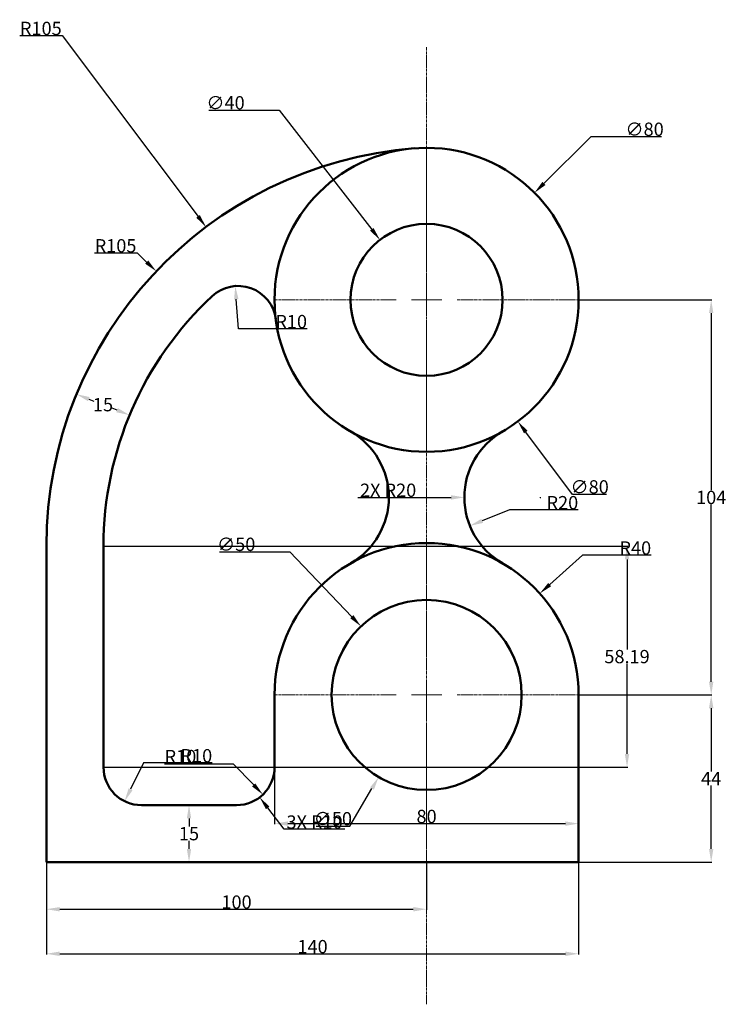
# Model space of a CAD drawing. Units: inches. Extents: x 53 to 239, y 0 to 259.
import ezdxf

# ---------------------------------------------------------------- set-up
doc = ezdxf.new("R2010")
doc.units = ezdxf.units.IN
doc.header["$MEASUREMENT"] = 0
doc.linetypes.add('CENTER2', pattern=[1.125, 0.75, -0.125, 0.125, -0.125])
for name, color, linetype, lineweight in [('M-CNTR', 4, 'CENTER2', 18), ('M-DIMS', 2, 'Continuous', 25), ('M-OUTL', 7, 'Continuous', 50)]:
    doc.layers.add(name, color=color, linetype=linetype, lineweight=lineweight)
doc.styles.get("Standard").update_dxf_attribs({"font": 'arial.ttf'})
doc.dimstyles.get("Standard").update_dxf_attribs({"dimtxt": 3.5, "dimasz": 3.5, "dimexe": 0.18, "dimexo": 0.0625, "dimgap": 0.09, "dimtad": 1, "dimtih": 1, "dimtoh": 1, "dimdec": 0, "dimzin": 0, "dimdsep": 46, "dimtxsty": 'Standard', "dimcen": 0.09, "dimadec": 0, "dimazin": 0, "dimtfac": 1, "dimtdec": 0, "dimtofl": 0, "dimtmove": 0, "dimatfit": 3, "dimfxl": 1, "dimtolj": 1, "dimtzin": 0, "dimarcsym": 0})

# ---------------------------------------------------------------- blocks, each defined once
blk = doc.blocks.new('*U1')
at = {"layer": 'M-CNTR', "color": 0, "transparency": 16777216}
for p, q in [((0, 8), (0, 40.12)), ((-40.12, 0), (-8, 0)), ((8, 0), (40.12, 0)), ((0, -40.12), (0, -8))]:
    blk.add_line(p, q, dxfattribs=at)
at = {"layer": 'M-CNTR', "color": 0, "linetype": 'Continuous', "transparency": 16777216}
for p, q in [((0, -4), (0, 4)), ((-4, 0), (4, 0))]:
    blk.add_line(p, q, dxfattribs=at)
blk = doc.blocks.new('*U2')
at = {"layer": 'M-CNTR', "color": 0, "transparency": 16777216}
for p, q in [((0, 8), (0, 40.12)), ((-40.12, 0), (-8, 0)), ((8, 0), (40.12, 0)), ((0, -40.12), (0, -8))]:
    blk.add_line(p, q, dxfattribs=at)
at = {"layer": 'M-CNTR', "color": 0, "linetype": 'Continuous', "transparency": 16777216}
for p, q in [((0, -4), (0, 4)), ((-4, 0), (4, 0))]:
    blk.add_line(p, q, dxfattribs=at)
blk = doc.blocks.new('*D3')
at = {"layer": 'Defpoints', "color": 0, "transparency": 16777216}
for p in [(188.49, 213.54), (131.72, 157.18)]:
    blk.add_point(p, dxfattribs=at)
at = {"layer": 'M-DIMS', "color": 0, "lineweight": -2, "transparency": 16777216}
for p, q in [((203.34, 228.29), (190.97, 216.01)), ((221.86, 228.29), (203.34, 228.29)), ((160.01, 185.36), (160.19, 185.36)), ((160.1, 185.27), (160.1, 185.45))]:
    blk.add_line(p, q, dxfattribs=at)
at = {"layer": 'M-DIMS', "color": 0, "transparency": 16777216}
blk.add_solid([(190.56, 216.42), (191.38, 215.59), (188.49, 213.54)], dxfattribs=at)
at = {"layer": 'M-DIMS', "color": 0, "transparency": 16777216, "insert": (217.45, 230.26), "char_height": 3.5, "attachment_point": 5}
blk.add_mtext('\\A1;∅80', dxfattribs=at)
blk = doc.blocks.new('*D4')
at = {"layer": 'Defpoints', "color": 0, "transparency": 16777216}
for p in [(147.83, 201.15), (172.38, 169.57)]:
    blk.add_point(p, dxfattribs=at)
at = {"layer": 'M-DIMS', "color": 0, "lineweight": -2, "transparency": 16777216}
for p, q in [((102.8, 235.24), (121.32, 235.24)), ((121.32, 235.24), (145.68, 203.91)), ((160.01, 185.36), (160.19, 185.36)), ((160.1, 185.27), (160.1, 185.45))]:
    blk.add_line(p, q, dxfattribs=at)
at = {"layer": 'M-DIMS', "color": 0, "transparency": 16777216}
blk.add_solid([(146.14, 204.27), (145.22, 203.55), (147.83, 201.15)], dxfattribs=at)
at = {"layer": 'M-DIMS', "color": 0, "transparency": 16777216, "insert": (107.21, 237.22), "char_height": 3.5, "attachment_point": 5}
blk.add_mtext('\\A1;∅40', dxfattribs=at)
blk = doc.blocks.new('*D5')
at = {"layer": 'Defpoints', "color": 0, "transparency": 16777216}
for p in [(142.83, 99.44), (177.37, 63.28)]:
    blk.add_point(p, dxfattribs=at)
at = {"layer": 'M-DIMS', "color": 0, "lineweight": -2, "transparency": 16777216}
for p, q in [((105.61, 119.03), (124.12, 119.03)), ((124.12, 119.03), (140.42, 101.97)), ((160.01, 81.36), (160.19, 81.36)), ((160.1, 81.27), (160.1, 81.45))]:
    blk.add_line(p, q, dxfattribs=at)
at = {"layer": 'M-DIMS', "color": 0, "transparency": 16777216}
blk.add_solid([(140.84, 102.37), (140, 101.57), (142.83, 99.44)], dxfattribs=at)
at = {"layer": 'M-DIMS', "color": 0, "transparency": 16777216, "insert": (110.01, 121.01), "char_height": 3.5, "attachment_point": 5}
blk.add_mtext('\\A1;∅50', dxfattribs=at)
blk = doc.blocks.new('*D6')
at = {"layer": 'Defpoints', "color": 0, "transparency": 16777216}
for p in [(109.78, 189), (110.5, 179.03)]:
    blk.add_point(p, dxfattribs=at)
at = {"layer": 'M-DIMS', "color": 0, "lineweight": -2, "transparency": 16777216}
for p, q in [((110.59, 177.76), (110.03, 185.51)), ((128.65, 177.76), (110.59, 177.76))]:
    blk.add_line(p, q, dxfattribs=at)
at = {"layer": 'M-DIMS', "color": 0, "transparency": 16777216}
blk.add_solid([(110.62, 185.55), (109.45, 185.47), (109.78, 189)], dxfattribs=at)
at = {"layer": 'M-DIMS', "color": 0, "transparency": 16777216, "insert": (124.48, 179.64), "char_height": 3.5, "attachment_point": 5}
blk.add_mtext('\\A1;R10', dxfattribs=at)
blk = doc.blocks.new('*D7')
at = {"layer": 'Defpoints', "color": 0, "transparency": 16777216}
for p in [(190.03, 133.36), (171.49, 125.88)]:
    blk.add_point(p, dxfattribs=at)
at = {"layer": 'M-DIMS', "color": 0, "lineweight": -2, "transparency": 16777216}
for p, q in [((181.93, 130.09), (174.73, 127.19)), ((199.99, 130.09), (181.93, 130.09))]:
    blk.add_line(p, q, dxfattribs=at)
at = {"layer": 'M-DIMS', "color": 0, "transparency": 16777216}
blk.add_solid([(174.51, 127.73), (174.95, 126.65), (171.49, 125.88)], dxfattribs=at)
at = {"layer": 'M-DIMS', "color": 0, "transparency": 16777216, "insert": (195.82, 131.97), "char_height": 3.5, "attachment_point": 5}
blk.add_mtext('\\A1;R20', dxfattribs=at)
blk = doc.blocks.new('*D8')
at = {"layer": 'Defpoints', "color": 0, "transparency": 16777216}
for p in [(189.87, 108.07), (160.1, 81.36)]:
    blk.add_point(p, dxfattribs=at)
at = {"layer": 'M-DIMS', "color": 0, "lineweight": -2, "transparency": 16777216}
for p, q in [((201.12, 118.17), (192.48, 110.41)), ((219.18, 118.17), (201.12, 118.17)), ((160.01, 81.36), (160.19, 81.36)), ((160.1, 81.27), (160.1, 81.45))]:
    blk.add_line(p, q, dxfattribs=at)
at = {"layer": 'M-DIMS', "color": 0, "transparency": 16777216}
blk.add_solid([(192.09, 110.84), (192.87, 109.98), (189.87, 108.07)], dxfattribs=at)
at = {"layer": 'M-DIMS', "color": 0, "transparency": 16777216, "insert": (215.01, 120.04), "char_height": 3.5, "attachment_point": 5}
blk.add_mtext('\\A1;R40', dxfattribs=at)
blk = doc.blocks.new('*D9')
at = {"layer": 'Defpoints', "color": 0, "transparency": 16777216}
for p in [(85.1, 62.36), (80.67, 53.39)]:
    blk.add_point(p, dxfattribs=at)
at = {"layer": 'M-DIMS', "color": 0, "lineweight": -2, "transparency": 16777216}
for p, q in [((85.66, 63.49), (82.22, 56.53)), ((103.72, 63.49), (85.66, 63.49))]:
    blk.add_line(p, q, dxfattribs=at)
at = {"layer": 'M-DIMS', "color": 0, "transparency": 16777216}
blk.add_solid([(81.7, 56.79), (82.74, 56.27), (80.67, 53.39)], dxfattribs=at)
at = {"layer": 'M-DIMS', "color": 0, "transparency": 16777216, "insert": (99.54, 65.37), "char_height": 3.5, "attachment_point": 5}
blk.add_mtext('\\A1;R10', dxfattribs=at)
blk = doc.blocks.new('*D10')
at = {"layer": 'Defpoints', "color": 0, "transparency": 16777216}
for p in [(110.1, 62.36), (117.04, 55.16)]:
    blk.add_point(p, dxfattribs=at)
at = {"layer": 'M-DIMS', "color": 0, "lineweight": -2, "transparency": 16777216}
for p, q in [((91.16, 63.27), (109.22, 63.27)), ((109.22, 63.27), (114.61, 57.68))]:
    blk.add_line(p, q, dxfattribs=at)
at = {"layer": 'M-DIMS', "color": 0, "transparency": 16777216}
blk.add_solid([(115.03, 58.08), (114.19, 57.27), (117.04, 55.16)], dxfattribs=at)
at = {"layer": 'M-DIMS', "color": 0, "transparency": 16777216, "insert": (95.34, 65.15), "char_height": 3.5, "attachment_point": 5}
blk.add_mtext('\\A1;R10', dxfattribs=at)
blk = doc.blocks.new('*D11')
at = {"layer": 'Defpoints', "color": 0, "transparency": 16777216}
for p in [(88.99, 192.89), (165.1, 120.55)]:
    blk.add_point(p, dxfattribs=at)
at = {"layer": 'M-DIMS', "color": 0, "lineweight": -2, "transparency": 16777216}
for p, q in [((72.72, 197.71), (83.92, 197.71)), ((83.92, 197.71), (86.46, 195.3)), ((165.01, 120.55), (165.19, 120.55)), ((165.1, 120.46), (165.1, 120.64))]:
    blk.add_line(p, q, dxfattribs=at)
at = {"layer": 'M-DIMS', "color": 0, "transparency": 16777216}
blk.add_solid([(86.86, 195.72), (86.05, 194.88), (88.99, 192.89)], dxfattribs=at)
at = {"layer": 'M-DIMS', "color": 0, "transparency": 16777216, "insert": (78.28, 199.59), "char_height": 3.5, "attachment_point": 5}
blk.add_mtext('\\A1;R105', dxfattribs=at)
blk = doc.blocks.new('*D12')
at = {"layer": 'Defpoints', "color": 0, "transparency": 16777216}
for p in [(67.39, 158.98), (67.99, 160.52), (81.35, 153.49)]:
    blk.add_point(p, dxfattribs=at)
at = {"layer": 'M-DIMS', "color": 0, "lineweight": -2, "transparency": 16777216}
for p, q in [((67.41, 159.04), (68.06, 160.69)), ((71.25, 159.24), (72.52, 158.73)), ((78.69, 156.31), (77.41, 156.81)), ((81.37, 153.55), (82.02, 155.2))]:
    blk.add_line(p, q, dxfattribs=at)
at = {"layer": 'M-DIMS', "color": 0, "transparency": 16777216}
for points in [[(71.46, 159.78), (71.03, 158.69), (67.99, 160.52)], [(78.91, 156.85), (78.48, 155.77), (81.95, 155.03)]]:
    blk.add_solid(points, dxfattribs=at)
at = {"layer": 'M-DIMS', "color": 0, "transparency": 16777216, "insert": (74.97, 157.77), "char_height": 3.5, "attachment_point": 5}
blk.add_mtext('\\A1;15', dxfattribs=at)
blk = doc.blocks.new('*D13')
at = {"layer": 'Defpoints', "color": 0, "transparency": 16777216}
for p in [(200.22, 185.36), (200.22, 81.36), (234.97, 81.36)]:
    blk.add_point(p, dxfattribs=at)
at = {"layer": 'M-DIMS', "color": 0, "lineweight": -2, "transparency": 16777216}
for p, q in [((200.28, 185.36), (235.15, 185.36)), ((234.97, 181.86), (234.97, 135.24)), ((234.97, 84.86), (234.97, 131.48)), ((200.28, 81.36), (235.15, 81.36))]:
    blk.add_line(p, q, dxfattribs=at)
at = {"layer": 'M-DIMS', "color": 0, "transparency": 16777216}
for points in [[(234.38, 181.86), (235.55, 181.86), (234.97, 185.36)], [(234.38, 84.86), (235.55, 84.86), (234.97, 81.36)]]:
    blk.add_solid(points, dxfattribs=at)
at = {"layer": 'M-DIMS', "color": 0, "transparency": 16777216, "insert": (234.97, 133.36), "char_height": 3.5, "attachment_point": 5}
blk.add_mtext('\\A1;104', dxfattribs=at)
blk = doc.blocks.new('*D14')
at = {"layer": 'Defpoints', "color": 0, "transparency": 16777216}
for p in [(200.22, 81.36), (200.1, 37.36), (234.97, 37.36)]:
    blk.add_point(p, dxfattribs=at)
at = {"layer": 'M-DIMS', "color": 0, "lineweight": -2, "transparency": 16777216}
for p, q in [((200.28, 81.36), (235.15, 81.36)), ((234.97, 77.86), (234.97, 61.2)), ((234.97, 40.86), (234.97, 57.52)), ((200.16, 37.36), (235.15, 37.36))]:
    blk.add_line(p, q, dxfattribs=at)
at = {"layer": 'M-DIMS', "color": 0, "transparency": 16777216}
for points in [[(234.38, 77.86), (235.55, 77.86), (234.97, 81.36)], [(234.38, 40.86), (235.55, 40.86), (234.97, 37.36)]]:
    blk.add_solid(points, dxfattribs=at)
at = {"layer": 'M-DIMS', "color": 0, "transparency": 16777216, "insert": (234.97, 59.36), "char_height": 3.5, "attachment_point": 5}
blk.add_mtext('\\A1;44', dxfattribs=at)
blk = doc.blocks.new('*D15')
at = {"layer": 'Defpoints', "color": 0, "transparency": 16777216}
for p in [(60.1, 37.36), (200.1, 37.36), (200.1, 13.24)]:
    blk.add_point(p, dxfattribs=at)
at = {"layer": 'M-DIMS', "color": 0, "lineweight": -2, "transparency": 16777216}
for p, q in [((60.1, 37.3), (60.1, 13.06)), ((200.1, 37.3), (200.1, 13.06)), ((63.6, 13.24), (196.6, 13.24))]:
    blk.add_line(p, q, dxfattribs=at)
at = {"layer": 'M-DIMS', "color": 0, "transparency": 16777216}
for points in [[(63.6, 13.83), (63.6, 12.66), (60.1, 13.24)], [(196.6, 13.83), (196.6, 12.66), (200.1, 13.24)]]:
    blk.add_solid(points, dxfattribs=at)
at = {"layer": 'M-DIMS', "color": 0, "transparency": 16777216, "insert": (130.1, 15.12), "char_height": 3.5, "attachment_point": 5}
blk.add_mtext('\\A1;140', dxfattribs=at)
blk = doc.blocks.new('*D16')
at = {"layer": 'Defpoints', "color": 0, "transparency": 16777216}
for p in [(60.1, 37.36), (160.1, 37.36), (160.1, 24.97)]:
    blk.add_point(p, dxfattribs=at)
at = {"layer": 'M-DIMS', "color": 0, "lineweight": -2, "transparency": 16777216}
for p, q in [((60.1, 37.3), (60.1, 24.79)), ((160.1, 37.3), (160.1, 24.79)), ((63.6, 24.97), (156.6, 24.97))]:
    blk.add_line(p, q, dxfattribs=at)
at = {"layer": 'M-DIMS', "color": 0, "transparency": 16777216}
for points in [[(63.6, 25.55), (63.6, 24.38), (60.1, 24.97)], [(156.6, 25.55), (156.6, 24.38), (160.1, 24.97)]]:
    blk.add_solid(points, dxfattribs=at)
at = {"layer": 'M-DIMS', "color": 0, "transparency": 16777216, "insert": (110.1, 26.85), "char_height": 3.5, "attachment_point": 5}
blk.add_mtext('\\A1;100', dxfattribs=at)
blk = doc.blocks.new('*D17')
at = {"layer": 'Defpoints', "color": 0, "transparency": 16777216}
for p in [(97.6, 52.36), (97.6, 52.36), (97.6, 37.36)]:
    blk.add_point(p, dxfattribs=at)
at = {"layer": 'M-DIMS', "color": 0, "lineweight": -2, "transparency": 16777216}
for p, q in [((97.66, 52.36), (97.78, 52.36)), ((97.6, 48.86), (97.6, 46.74)), ((97.6, 40.86), (97.6, 42.98)), ((97.66, 37.36), (97.78, 37.36))]:
    blk.add_line(p, q, dxfattribs=at)
at = {"layer": 'M-DIMS', "color": 0, "transparency": 16777216}
for points in [[(97.02, 48.86), (98.18, 48.86), (97.6, 52.36)], [(97.02, 40.86), (98.18, 40.86), (97.6, 37.36)]]:
    blk.add_solid(points, dxfattribs=at)
at = {"layer": 'M-DIMS', "color": 0, "transparency": 16777216, "insert": (97.6, 44.86), "char_height": 3.5, "attachment_point": 5}
blk.add_mtext('\\A1;15', dxfattribs=at)
blk = doc.blocks.new('*D18')
at = {"layer": 'Defpoints', "color": 0, "transparency": 16777216}
for p in [(120.1, 62.36), (200.1, 62.36), (200.1, 47.5)]:
    blk.add_point(p, dxfattribs=at)
at = {"layer": 'M-DIMS', "color": 0, "lineweight": -2, "transparency": 16777216}
for p, q in [((120.1, 62.3), (120.1, 47.32)), ((200.1, 62.3), (200.1, 47.32)), ((123.6, 47.5), (196.6, 47.5))]:
    blk.add_line(p, q, dxfattribs=at)
at = {"layer": 'M-DIMS', "color": 0, "transparency": 16777216}
for points in [[(123.6, 48.08), (123.6, 46.92), (120.1, 47.5)], [(196.6, 48.08), (196.6, 46.92), (200.1, 47.5)]]:
    blk.add_solid(points, dxfattribs=at)
at = {"layer": 'M-DIMS', "color": 0, "transparency": 16777216, "insert": (160.1, 49.38), "char_height": 3.5, "attachment_point": 5}
blk.add_mtext('\\A1;80', dxfattribs=at)
blk = doc.blocks.new('*D19')
at = {"layer": 'Defpoints', "color": 0, "transparency": 16777216}
for p in [(75.1, 120.55), (212.83, 120.55), (75.1, 62.36)]:
    blk.add_point(p, dxfattribs=at)
at = {"layer": 'M-DIMS', "color": 0, "lineweight": -2, "transparency": 16777216}
for p, q in [((75.16, 120.55), (213.01, 120.55)), ((212.83, 117.05), (212.83, 93.33)), ((212.83, 65.86), (212.83, 89.58)), ((75.16, 62.36), (213.01, 62.36))]:
    blk.add_line(p, q, dxfattribs=at)
at = {"layer": 'M-DIMS', "color": 0, "transparency": 16777216}
for points in [[(212.25, 117.05), (213.41, 117.05), (212.83, 120.55)], [(212.25, 65.86), (213.41, 65.86), (212.83, 62.36)]]:
    blk.add_solid(points, dxfattribs=at)
at = {"layer": 'M-DIMS', "color": 0, "transparency": 16777216, "insert": (212.83, 91.46), "char_height": 3.5, "attachment_point": 5}
blk.add_mtext('\\A1;58.19', dxfattribs=at)
blk = doc.blocks.new('*D20')
at = {"layer": 'Defpoints', "color": 0, "transparency": 16777216}
for p in [(102.08, 204.53), (165.1, 120.55)]:
    blk.add_point(p, dxfattribs=at)
at = {"layer": 'M-DIMS', "color": 0, "lineweight": -2, "transparency": 16777216}
for p, q in [((53.06, 254.92), (64.26, 254.92)), ((64.26, 254.92), (99.97, 207.33)), ((165.01, 120.55), (165.19, 120.55)), ((165.1, 120.46), (165.1, 120.64))]:
    blk.add_line(p, q, dxfattribs=at)
at = {"layer": 'M-DIMS', "color": 0, "transparency": 16777216}
blk.add_solid([(100.44, 207.68), (99.51, 206.98), (102.08, 204.53)], dxfattribs=at)
at = {"layer": 'M-DIMS', "color": 0, "transparency": 16777216, "insert": (58.62, 256.8), "char_height": 3.5, "attachment_point": 5}
blk.add_mtext('\\A1;R105', dxfattribs=at)
blk = doc.blocks.new('*D21')
at = {"layer": 'Defpoints', "color": 0, "transparency": 16777216}
for p in [(136.1, 217.36), (184.1, 153.36)]:
    blk.add_point(p, dxfattribs=at)
at = {"layer": 'M-DIMS', "color": 0, "lineweight": -2, "transparency": 16777216}
for p, q in [((160.01, 185.36), (160.19, 185.36)), ((160.1, 185.27), (160.1, 185.45)), ((198.5, 134.16), (186.2, 150.56)), ((207.4, 134.16), (198.5, 134.16))]:
    blk.add_line(p, q, dxfattribs=at)
at = {"layer": 'M-DIMS', "color": 0, "transparency": 16777216}
blk.add_solid([(186.67, 150.91), (185.73, 150.21), (184.1, 153.36)], dxfattribs=at)
at = {"layer": 'M-DIMS', "color": 0, "transparency": 16777216, "insert": (202.99, 136.13), "char_height": 3.5, "attachment_point": 5}
blk.add_mtext('\\A1;∅80', dxfattribs=at)
blk = doc.blocks.new('*D22')
at = {"layer": 'Defpoints', "color": 0, "transparency": 16777216}
for p in [(172.7, 102.95), (147.5, 59.77)]:
    blk.add_point(p, dxfattribs=at)
at = {"layer": 'M-DIMS', "color": 0, "lineweight": -2, "transparency": 16777216}
for p, q in [((160.01, 81.36), (160.19, 81.36)), ((160.1, 81.27), (160.1, 81.45)), ((139.94, 46.81), (145.73, 56.75)), ((131.04, 46.81), (139.94, 46.81))]:
    blk.add_line(p, q, dxfattribs=at)
at = {"layer": 'M-DIMS', "color": 0, "transparency": 16777216}
blk.add_solid([(145.23, 57.04), (146.24, 56.45), (147.5, 59.77)], dxfattribs=at)
at = {"layer": 'M-DIMS', "color": 0, "transparency": 16777216, "insert": (135.44, 48.79), "char_height": 3.5, "attachment_point": 5}
blk.add_mtext('\\A1;∅50', dxfattribs=at)
blk = doc.blocks.new('*D23')
at = {"layer": 'Defpoints', "color": 0, "transparency": 16777216}
for p in [(170.03, 133.36), (190.03, 133.36)]:
    blk.add_point(p, dxfattribs=at)
at = {"layer": 'M-DIMS', "color": 0, "lineweight": -2, "transparency": 16777216}
for p, q in [((142.01, 133.36), (158.03, 133.36)), ((158.03, 133.36), (166.53, 133.36)), ((189.94, 133.36), (190.12, 133.36)), ((190.03, 133.27), (190.03, 133.45))]:
    blk.add_line(p, q, dxfattribs=at)
at = {"layer": 'M-DIMS', "color": 0, "transparency": 16777216}
blk.add_solid([(166.53, 133.94), (166.53, 132.78), (170.03, 133.36)], dxfattribs=at)
at = {"layer": 'M-DIMS', "color": 0, "transparency": 16777216, "insert": (149.98, 135.24), "char_height": 3.5, "attachment_point": 5}
blk.add_mtext('\\A1;2X R20', dxfattribs=at)
blk = doc.blocks.new('*D24')
at = {"layer": 'Defpoints', "color": 0, "transparency": 16777216}
for p in [(110.1, 62.36), (116.18, 54.42)]:
    blk.add_point(p, dxfattribs=at)
at = {"layer": 'M-DIMS', "color": 0, "lineweight": -2, "transparency": 16777216}
for p, q in [((110.01, 62.36), (110.19, 62.36)), ((110.1, 62.27), (110.1, 62.45)), ((122.62, 46.03), (118.31, 51.64)), ((138.58, 46.03), (122.62, 46.03))]:
    blk.add_line(p, q, dxfattribs=at)
at = {"layer": 'M-DIMS', "color": 0, "transparency": 16777216}
blk.add_solid([(118.77, 52), (117.85, 51.29), (116.18, 54.42)], dxfattribs=at)
at = {"layer": 'M-DIMS', "color": 0, "transparency": 16777216, "insert": (130.64, 47.91), "char_height": 3.5, "attachment_point": 5}
blk.add_mtext('\\A1;3X R10', dxfattribs=at)

msp = doc.modelspace()

# ---------------------------------------------------------------- linework, layer by layer
at = {"layer": 'M-CNTR'}
msp.add_line((160.101, 251.886), (160.101, -0.057), dxfattribs=at)
at = {"layer": 'M-OUTL'}
for p, q in [((60.101, 120.552), (60.101, 37.36)), ((75.101, 62.36), (75.101, 120.552)), ((120.101, 81.36), (120.101, 62.36)), ((200.101, 81.36), (200.101, 37.36)), ((85.101, 52.36), (110.101, 52.36)), ((60.101, 37.36), (200.101, 37.36))]:
    msp.add_line(p, q, dxfattribs=at)
for centre, radius in [((160.101, 185.36), 40), ((160.101, 185.36), 40), ((160.101, 185.36), 20), ((160.101, 81.36), 25)]:
    msp.add_circle(centre, radius, dxfattribs=at)
for centre, radius, start, end in [((165.101, 120.552), 105, 94.41173, 180), ((110.504, 179.026), 10, 7.27771, 133.03656), ((165.101, 120.552), 90, 133.03656, 180), ((130.167, 133.36), 20, 299.92643, 60.07357), ((190.034, 133.36), 20, 119.92643, 240.07357), ((160.101, 81.36), 40, 0, 180), ((85.101, 62.36), 10, 180, 270), ((110.101, 62.36), 10, 270, 0)]:
    msp.add_arc(centre, radius, start, end, dxfattribs=at)

# ---------------------------------------------------------------- block references
at = {"layer": 'M-CNTR'}
for name, p in [('*U1', (160.101, 185.36)), ('*U2', (160.101, 81.36))]:
    msp.add_blockref(name, p, dxfattribs=at)

# ---------------------------------------------------------------- dimensions: what is measured, and where the dimension line sits
at = {"layer": 'M-DIMS'}
for center, mpoint, override, picture, middle in [((165.101, 120.552), (102.075, 204.533), {"dimdec": 0, "dimlfac": 1, "dimrnd": 0, "dimzin": 0, "dimdsep": 46, "dimlunit": 2}, '*D20', (58.615, 254.922)), ((110.504, 179.026), (109.783, 189), {"dimclrd": 0, "dimclre": 0, "dimclrt": 0}, '*D6', (124.478, 177.764)), ((190.034, 133.36), (171.485, 125.88), {"dimclrd": 0, "dimclre": 0, "dimclrt": 0}, '*D7', (195.817, 130.093)), ((160.101, 81.36), (189.873, 108.073), {"dimclrd": 0, "dimclre": 0, "dimclrt": 0}, '*D8', (215.008, 118.168)), ((85.101, 62.36), (80.671, 53.395), {"dimclrd": 0, "dimclre": 0, "dimclrt": 0}, '*D9', (99.545, 63.494)), ((110.101, 62.36), (117.038, 55.157), {"dimclrd": 0, "dimclre": 0, "dimclrt": 0}, '*D10', (95.339, 63.271))]:
    dim = msp.add_radius_dim(center=center, mpoint=mpoint, dimstyle='Standard', override=override, dxfattribs=at)
    dim.commit()
    dim.dimension.update_dxf_attribs({"geometry": picture, "text_midpoint": middle, "dimtype": 164})
for p1, p2, override, picture, middle in [((172.376, 169.57), (147.825, 201.149), {"dimclrd": 0, "dimclre": 0, "dimclrt": 0}, '*D4', (107.205, 235.244)), ((131.715, 157.177), (188.486, 213.543), {"dimclrd": 0, "dimclre": 0, "dimclrt": 0}, '*D3', (217.451, 228.288)), ((136.101, 217.36), (184.1, 153.36), {"dimdec": 0, "dimlfac": 1, "dimrnd": 0, "dimzin": 0, "dimdsep": 46, "dimlunit": 2}, '*D21', (202.995, 134.159)), ((177.367, 63.28), (142.835, 99.44), {"dimclrd": 0, "dimclre": 0, "dimclrt": 0}, '*D5', (110.012, 119.031)), ((172.703, 102.951), (147.499, 59.768), {"dimdec": 0, "dimlfac": 1, "dimrnd": 0, "dimzin": 0, "dimdsep": 46, "dimlunit": 2}, '*D22', (135.443, 46.813))]:
    dim = msp.add_diameter_dim_2p(p1=p1, p2=p2, dimstyle='Standard', override=override, dxfattribs=at)
    dim.commit()
    dim.dimension.update_dxf_attribs({"geometry": picture, "text_midpoint": middle, "dimtype": 163})
dim = msp.add_radius_dim(center=(165.101, 120.552), mpoint=(88.993, 192.889), dimstyle='Standard', override={"dimclrd": 0, "dimclre": 0, "dimclrt": 0}, dxfattribs=at)
dim.commit()
dim.dimension.update_dxf_attribs({"geometry": '*D11', "text_midpoint": (78.275, 199.589)})
for base, p1, p2, override, picture, middle in [((234.965, 81.36), (200.221, 185.36), (200.221, 81.36), {"dimclrd": 0, "dimclre": 0, "dimclrt": 0}, '*D13', (234.965, 133.36)), ((212.831, 120.552), (75.101, 62.36), (75.101, 120.552), {"dimdec": 2, "dimlfac": 1, "dimrnd": 0, "dimzin": 0, "dimdsep": 46, "dimlunit": 2}, '*D19', (212.831, 91.456)), ((234.965, 37.36), (200.221, 81.36), (200.101, 37.36), {"dimclrd": 0, "dimclre": 0, "dimclrt": 0, "dimtmove": 1}, '*D14', (234.965, 59.36)), ((97.601, 52.36), (97.601, 37.36), (97.601, 52.36), {"dimclrd": 0, "dimclre": 0, "dimclrt": 0}, '*D17', (97.601, 44.86))]:
    dim = msp.add_linear_dim(base=base, p1=p1, p2=p2, angle=90, dimstyle='Standard', override=override, dxfattribs=at)
    dim.commit()
    dim.dimension.update_dxf_attribs({"geometry": picture, "text_midpoint": middle})
dim = msp.add_aligned_dim(p1=(81.346, 153.493), p2=(67.386, 158.983), distance=-1.649, dimstyle='Standard', override={"dimclrd": 0, "dimclre": 0, "dimclrt": 0}, dxfattribs=at)
dim.commit()
dim.dimension.update_dxf_attribs({"geometry": '*D12', "text_midpoint": (74.97, 157.773)})
dim = msp.add_radius_dim(center=(190.034, 133.36), mpoint=(170.034, 133.36), text='2X <>', dimstyle='Standard', override={"dimdec": 0, "dimlfac": 1, "dimrnd": 0, "dimzin": 0, "dimdsep": 46, "dimlunit": 2}, dxfattribs=at)
dim.commit()
dim.dimension.update_dxf_attribs({"geometry": '*D23', "text_midpoint": (158.034, 133.36), "dimtype": 164})
dim = msp.add_radius_dim(center=(110.101, 62.36), mpoint=(116.183, 54.422), text='3X <>', dimstyle='Standard', override={"dimdec": 0, "dimlfac": 1, "dimrnd": 0, "dimzin": 0, "dimdsep": 46, "dimlunit": 2}, dxfattribs=at)
dim.commit()
dim.dimension.update_dxf_attribs({"geometry": '*D24', "text_midpoint": (130.641, 47.905)})
for base, p1, p2, picture, middle in [((200.101, 47.499), (120.101, 62.36), (200.101, 62.36), '*D18', (160.101, 49.376)), ((200.101, 13.243), (60.101, 37.36), (200.101, 37.36), '*D15', (130.101, 15.12)), ((160.101, 24.968), (60.101, 37.36), (160.101, 37.36), '*D16', (110.101, 26.845))]:
    dim = msp.add_linear_dim(base=base, p1=p1, p2=p2, dimstyle='Standard', override={"dimclrd": 0, "dimclre": 0, "dimclrt": 0}, dxfattribs=at)
    dim.commit()
    dim.dimension.update_dxf_attribs({"geometry": picture, "text_midpoint": middle})

doc.saveas('drawing.dxf')
